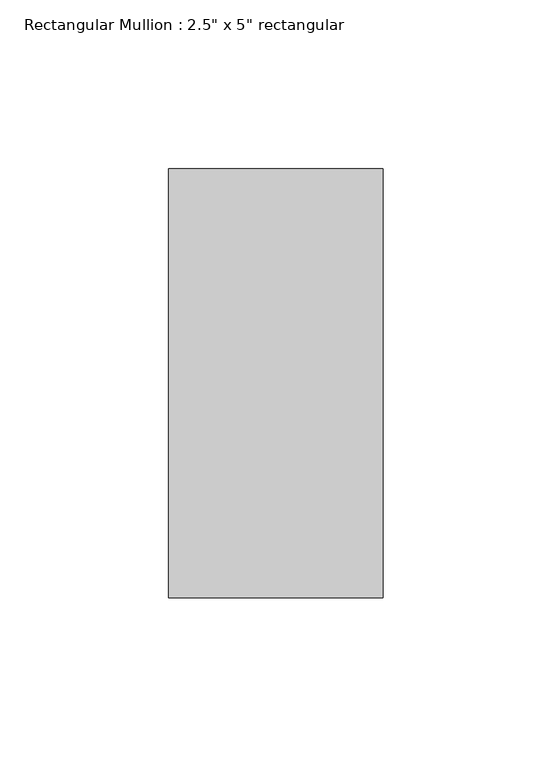
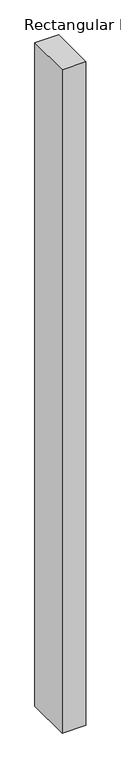
"""IFC4 building model written with IfcOpenShell, lengths in millimetres: member geometry."""

from ifc_helpers import new_model, si_unit, frame, origin, place, context, project, spatial, polyline, outline, extrude, source, transform, mapped, element, save


def member_c9c2ffa2(model_context):
    return source(origin(), model_context, "Body", "SweptSolid", [
        extrude(outline(polyline([(0.0, 63.5), (0.0, -63.5), (-63.5, -63.5), (-63.5, 63.5), (0.0, 63.5)])), frame((0.0, 0.0, -1887.2910101), z_axis=(0.0, 0.0, 1.0), x_axis=(1.0, 0.0, 0.0)), (0.0, 0.0, 1.0), 1887.2910101),
    ])


if __name__ == "__main__":
    model = new_model("IFC4")
    model_context = context("Model", 3, world=origin())
    ifc_project = project(units=[si_unit("LENGTHUNIT", "METRE", prefix="MILLI")], contexts=[model_context])
    site = spatial("IfcSite", under=ifc_project)
    building = spatial("IfcBuilding", under=site)
    placement = place(None, origin())
    member_shape = member_c9c2ffa2(model_context)
    element("IfcMember", 1, ObjectType="Rectangular Mullion : 2.5\" x 5\" rectangular", at=placement, inside=building, context=model_context, shape_type="MappedRepresentation", body=[
        mapped(member_shape, transform((0.0, 0.0, 0.0), x_axis=(1.0, 0.0, 0.0), y_axis=(0.0, 1.0, 0.0), z_axis=(0.0, 0.0, 1.0))),
    ])
    save(model, "model.ifc")

# Revit data of these elements
# Type "Rectangular Mullion : 2.5\" x 5\" rectangular"
#   built-in parameter 1007304 = 0.416667 (stored number, unit not read)
#   built-in parameter 1007301 = 0.104167 (stored number, unit not read)
#   built-in parameter 1007300 = 0.104167 (stored number, unit not read)
# Element 1 (IfcMember, "Rectangular Mullion : 2.5\" x 5\" rectangular")
#   Materials on its faces: "Aluminum"
# Materials
#   "Aluminum": class "Metal", colour RGB 247 247 247, transparency 0, Description = "Aluminum 6061", Cost = 0
